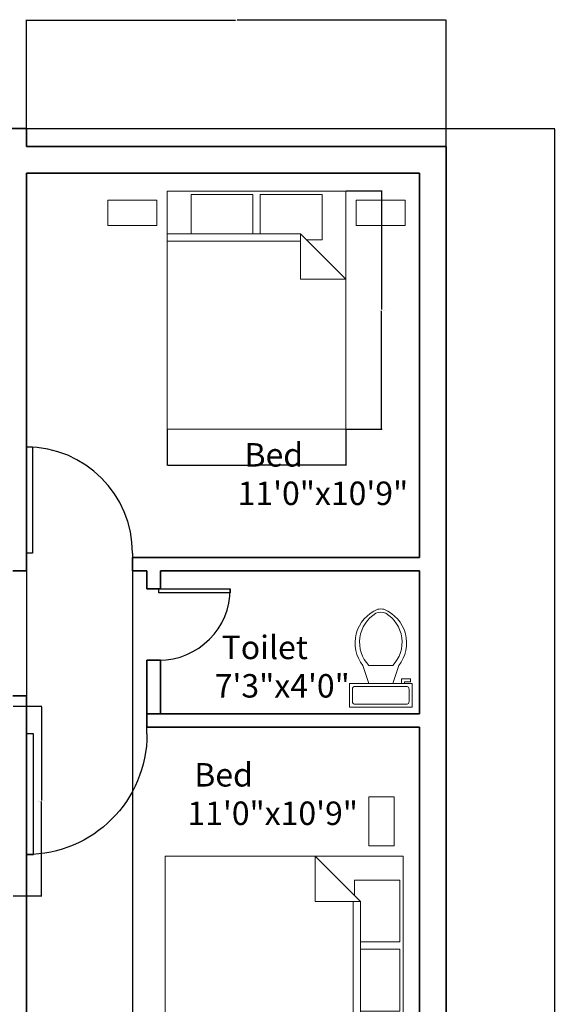
# Model space of a CAD drawing. Units: inches. Extents: x 108 to 613, y 1573 to 2319.
# Tile 11 of 11: x 434 to 613, y 1989 to 2319. Entities that reach past the tile are written whole.
import ezdxf

# ---------------------------------------------------------------- set-up
doc = ezdxf.new("R2010")
doc.units = ezdxf.units.IN
for name, color, linetype, lineweight in [('A-ANNO-DIMS', 2, 'Continuous', 18), ('A-AREA-IDEN', 3, 'Continuous', 18), ('A-FLOR-FIXT', 2, 'Continuous', 18), ('door', 4, 'Continuous', 25), ('furniture', 2, 'Continuous', 18), ('wall', 6, 'Continuous', 35)]:
    doc.layers.add(name, color=color, linetype=linetype, lineweight=lineweight)
doc.styles.get("Standard").update_dxf_attribs({"font": 'arial.ttf'})
doc.dimstyles.get("Standard").update_dxf_attribs({"dimtxt": 0.18, "dimasz": 0.18, "dimexe": 0.18, "dimexo": 0.0625, "dimgap": 0.09, "dimtad": 0, "dimtih": 1, "dimtoh": 1, "dimdec": 4, "dimzin": 0, "dimdsep": 46, "dimtxsty": 'Standard', "dimcen": 0.09, "dimadec": 0, "dimazin": 0, "dimtfac": 1, "dimtdec": 4, "dimtofl": 0, "dimtmove": 0, "dimatfit": 3, "dimfxl": 1, "dimtolj": 1, "dimtzin": 0, "dimarcsym": 0})

# ---------------------------------------------------------------- blocks, each defined once
blk = doc.blocks.new('*U2')
for p, q in [((0, 0), (0, -5)), ((30, 0), (30, -5))]:
    blk.add_line(p, q)
blk.add_lwpolyline([(0, 0), (0, 30), (1.75, 30), (1.75, 0)], close=True)
blk.add_arc((0, 0), 30, 0, 90)
blk = doc.blocks.new('Bed - Queen')
for p, q in [((0, -80.00003), (0, 0)), ((0, 0), (59.99999, 0)), ((59.99999, 0), (59.99999, -80.00003)), ((7.99999, -1.2), (28.79998, -1.2)), ((7.99999, -14.4), (7.99999, -1.2)), ((28.79998, -1.2), (28.79998, -14.4)), ((31.19999, -1.2), (51.99999, -1.2)), ((31.19999, -14.4), (31.19999, -1.2)), ((51.99999, -1.2), (51.99999, -16.4)), ((0, -14.4), (44.8, -14.4)), ((59.99999, -29.6), (44.8, -14.4)), ((44.8, -14.4), (44.8, -29.6)), ((51.99999, -16.4), (46.79936, -16.4)), ((44.8, -16.8), (0, -16.8)), ((44.8, -29.6), (59.99999, -29.6)), ((59.99999, -80.00003), (0, -80.00003))]:
    blk.add_line(p, q)
blk = doc.blocks.new('Toilet - top')
for p, q in [((9.5, -6), (9.5, -2)), ((-10, -8.5), (-8, -8.5)), ((-10, -9.5), (-10, -8.5)), ((-7, -9.5), (-10, -9.5)), ((-8, -8.5), (-8, -8)), ((-7, -8), (-7, -9.5)), ((-4, -8), (-6, -14)), ((4, -8), (6, -14)), ((4, -14), (-4, -14))]:
    blk.add_line(p, q)
blk.add_lwpolyline([(10.5, -8), (10.5, 0), (-10.5, 0), (-10.5, -8)], close=True)
for points in [[(-9.5, -2), (-9.5, -6)], [(8.5, -1), (-8.5, -1)], [(-8.5, -7), (8.5, -7)]]:
    blk.add_lwpolyline(points)
for centre, radius, start, end in [((-8.62, -1.88), 0.884, 81.8699, 188.1301), ((8.62, -1.88), 0.884, 351.8699, 98.1301), ((-8.62, -6.12), 0.884, 171.8699, 278.1301), ((8.62, -6.12), 0.884, 261.8699, 8.1301), ((3.52, -21.58), 12.17, 141.4691, 247.9714), ((4.2, -21.82), 11.33, 136.3677, 238.9468), ((-3.52, -21.58), 12.17, 292.0284, 38.5307), ((-4.2, -21.82), 11.33, 301.053, 43.6321), ((0, -27.88), 4, 245.7318, 294.2682), ((0, -29), 4, 254.8605, 285.1395)]:
    blk.add_arc(centre, radius, start, end)
blk = doc.blocks.new('NIGHTSTAND')
blk.add_lwpolyline([(0, 8.48), (16.5, 8.48), (16.5, 0), (0, 0)], close=True)
blk = doc.blocks.new('*D21')
at = {"layer": 'A-ANNO-DIMS', "color": 0, "lineweight": -2, "transparency": 16777216}
for p, q in [((543.14, 2261.64), (555.26, 2261.64)), ((555.08, 2261.46), (555.08, 2221.82)), ((555.08, 2181.82), (555.08, 2221.45)), ((543.14, 2181.64), (555.26, 2181.64))]:
    blk.add_line(p, q, dxfattribs=at)
at = {"layer": 'A-ANNO-DIMS', "color": 0, "transparency": 16777216}
for points in [[(555.05, 2261.46), (555.11, 2261.46), (555.08, 2261.64)], [(555.05, 2181.82), (555.11, 2181.82), (555.08, 2181.64)]]:
    blk.add_solid(points, dxfattribs=at)
at = {"layer": 'Defpoints', "color": 0, "transparency": 16777216}
for p in [(543.08, 2261.64), (555.08, 2261.64), (543.08, 2181.64)]:
    blk.add_point(p, dxfattribs=at)
at = {"layer": 'A-ANNO-DIMS', "color": 0, "transparency": 16777216, "insert": (555.08, 2221.64), "char_height": 0.18, "attachment_point": 5}
blk.add_mtext('\\A1;QUEEN BED 80 TYP.', dxfattribs=at)
blk = doc.blocks.new('*D22')
at = {"layer": 'A-ANNO-DIMS', "color": 0, "lineweight": -2, "transparency": 16777216}
for p, q in [((483.08, 2181.57), (483.08, 2169.46)), ((543.08, 2181.57), (543.08, 2169.46)), ((483.26, 2169.64), (512.55, 2169.64)), ((542.9, 2169.64), (513.61, 2169.64))]:
    blk.add_line(p, q, dxfattribs=at)
at = {"layer": 'A-ANNO-DIMS', "color": 0, "transparency": 16777216}
for points in [[(483.26, 2169.67), (483.26, 2169.61), (483.08, 2169.64)], [(542.9, 2169.67), (542.9, 2169.61), (543.08, 2169.64)]]:
    blk.add_solid(points, dxfattribs=at)
at = {"layer": 'Defpoints', "color": 0, "transparency": 16777216}
for p in [(483.08, 2181.64), (543.08, 2181.64), (543.08, 2169.64)]:
    blk.add_point(p, dxfattribs=at)
at = {"layer": 'A-ANNO-DIMS', "color": 0, "transparency": 16777216, "insert": (513.08, 2169.64), "char_height": 0.18, "attachment_point": 5}
blk.add_mtext('\\A1;60 TYP.', dxfattribs=at)
blk = doc.blocks.new('*D31')
at = {"layer": 'A-ANNO-DIMS', "color": 0, "lineweight": -2, "transparency": 16777216}
for p, q in [((431.34, 2088.69), (441, 2088.69)), ((440.82, 2088.51), (440.82, 2057.05)), ((440.82, 2025.21), (440.82, 2056.68)), ((431.34, 2025.03), (441, 2025.03))]:
    blk.add_line(p, q, dxfattribs=at)
at = {"layer": 'A-ANNO-DIMS', "color": 0, "transparency": 16777216}
for points in [[(440.79, 2088.51), (440.85, 2088.51), (440.82, 2088.69)], [(440.79, 2025.21), (440.85, 2025.21), (440.82, 2025.03)]]:
    blk.add_solid(points, dxfattribs=at)
at = {"layer": 'Defpoints', "color": 0, "transparency": 16777216}
for p in [(431.28, 2088.69), (440.82, 2088.69), (431.28, 2025.03)]:
    blk.add_point(p, dxfattribs=at)
at = {"layer": 'A-ANNO-DIMS', "color": 0, "transparency": 16777216, "insert": (440.82, 2056.86), "char_height": 0.18, "attachment_point": 5}
blk.add_mtext('\\A1;3-SEAT SOFA 64 TYP.', dxfattribs=at)
blk = doc.blocks.new('*D40')
at = {"layer": 'A-ANNO-DIMS', "color": 0, "lineweight": -2, "transparency": 16777216}
for p, q in [((435.84, 2282.61), (613.31, 2282.61)), ((613.13, 2282.43), (613.13, 1951.37)), ((613.13, 1619.94), (613.13, 1951.01)), ((435.84, 1619.76), (613.31, 1619.76))]:
    blk.add_line(p, q, dxfattribs=at)
at = {"layer": 'A-ANNO-DIMS', "color": 0, "transparency": 16777216}
for points in [[(613.1, 2282.43), (613.16, 2282.43), (613.13, 2282.61)], [(613.1, 1619.94), (613.16, 1619.94), (613.13, 1619.76)]]:
    blk.add_solid(points, dxfattribs=at)
at = {"layer": 'Defpoints', "color": 0, "transparency": 16777216}
for p in [(435.78, 2282.61), (613.13, 2282.61), (435.78, 1619.76)]:
    blk.add_point(p, dxfattribs=at)
at = {"layer": 'A-ANNO-DIMS', "color": 0, "transparency": 16777216, "insert": (613.13, 1951.19), "char_height": 0.18, "attachment_point": 5}
blk.add_mtext('\\A1;662.8', dxfattribs=at)
blk = doc.blocks.new('*D42')
at = {"layer": 'A-ANNO-DIMS', "color": 0, "lineweight": -2, "transparency": 16777216}
for p, q in [((435.78, 2282.67), (435.78, 2319.14)), ((435.96, 2318.96), (506.01, 2318.96)), ((576.6, 2318.96), (506.54, 2318.96)), ((576.78, 2276.67), (576.78, 2319.14))]:
    blk.add_line(p, q, dxfattribs=at)
at = {"layer": 'A-ANNO-DIMS', "color": 0, "transparency": 16777216}
for points in [[(435.96, 2318.99), (435.96, 2318.93), (435.78, 2318.96)], [(576.6, 2318.99), (576.6, 2318.93), (576.78, 2318.96)]]:
    blk.add_solid(points, dxfattribs=at)
at = {"layer": 'Defpoints', "color": 0, "transparency": 16777216}
for p in [(576.78, 2318.96), (435.78, 2282.61), (576.78, 2276.61)]:
    blk.add_point(p, dxfattribs=at)
at = {"layer": 'A-ANNO-DIMS', "color": 0, "transparency": 16777216, "insert": (506.28, 2318.96), "char_height": 0.18, "attachment_point": 5}
blk.add_mtext('\\A1;141', dxfattribs=at)
blk = doc.blocks.new('*D50')
at = {"layer": 'A-ANNO-DIMS', "color": 0, "lineweight": -2, "transparency": 16777216}
for p, q in [((471.43, 2138.55), (471.43, 1583.23)), ((435.78, 2137.91), (435.78, 1583.23)), ((435.96, 1583.41), (453.21, 1583.41)), ((471.25, 1583.41), (454, 1583.41))]:
    blk.add_line(p, q, dxfattribs=at)
at = {"layer": 'A-ANNO-DIMS', "color": 0, "transparency": 16777216}
for points in [[(435.96, 1583.44), (435.96, 1583.38), (435.78, 1583.41)], [(471.25, 1583.44), (471.25, 1583.38), (471.43, 1583.41)]]:
    blk.add_solid(points, dxfattribs=at)
at = {"layer": 'Defpoints', "color": 0, "transparency": 16777216}
for p in [(471.43, 2138.61), (435.78, 2137.98), (471.43, 1583.41)]:
    blk.add_point(p, dxfattribs=at)
at = {"layer": 'A-ANNO-DIMS', "color": 0, "transparency": 16777216, "insert": (453.6, 1583.41), "char_height": 0.18, "attachment_point": 5}
blk.add_mtext('\\A1;35.66', dxfattribs=at)

msp = doc.modelspace()

# ---------------------------------------------------------------- linework, layer by layer
at = {"layer": 'wall'}
for p, q in [((294.7753, 2282.6125), (435.7753, 2282.6125)), ((435.7753, 2276.6125), (435.7753, 2282.6125)), ((435.7753, 2276.6125), (576.7753, 2276.6125)), ((576.7753, 2276.6125), (576.7753, 1628.6125)), ((435.7753, 2267.6125), (435.7753, 2134.1125)), ((435.7753, 2267.6125), (567.7753, 2267.6125)), ((567.7753, 2267.6125), (567.7753, 2138.6125)), ((471.4334, 2138.6125), (567.7753, 2138.6125)), ((471.4334, 2138.6125), (471.4334, 2134.1125)), ((431.2753, 2134.1125), (435.7753, 2134.1125)), ((471.4334, 2134.1125), (476.2753, 2134.1125)), ((476.2753, 2134.1125), (476.2753, 2128.1125)), ((480.7753, 2134.1125), (480.7753, 2128.1125)), ((480.7753, 2134.1125), (567.7753, 2134.1125)), ((567.7753, 2134.1125), (567.7753, 2086.1125)), ((476.2753, 2128.1125), (480.7753, 2128.1125)), ((476.2753, 2104.1125), (480.7753, 2104.1125)), ((476.2753, 2104.1125), (476.2753, 2081.6125)), ((480.7753, 2104.1125), (480.7753, 2086.1125)), ((431.2753, 2092.1125), (435.7753, 2092.1125)), ((435.7753, 2092.1125), (435.7753, 1814.6125)), ((476.2753, 2086.1125), (567.7753, 2086.1125)), ((476.2753, 2081.6125), (567.7753, 2081.6125)), ((567.7753, 2081.6125), (567.7753, 1819.1125))]:
    msp.add_line(p, q, dxfattribs=at)

# ---------------------------------------------------------------- block references
at = {"layer": 'A-FLOR-FIXT', "rotation": 180}
msp.add_blockref('Toilet - top', (554.823, 2088.347), dxfattribs=at)
at = {"layer": 'door', "xscale": 1.188601040412397, "yscale": 1.188601040412397, "zscale": 1.188601040412397}
msp.add_blockref('*U2', (435.7753, 2140.0555), dxfattribs=at)
at = {"layer": 'door'}
for p, xscale, yscale, zscale, rotation in [((480.2753, 2128.1125), 0.8, 0.8, 0.8, 270), ((435.7753, 2079.3625), -1.350000000000012, 1.350000000000012, 1.350000000000012, 180)]:
    msp.add_blockref('*U2', p, dxfattribs=dict(at, xscale=xscale, yscale=yscale, zscale=zscale, rotation=rotation))
at = {"layer": 'furniture'}
for name, p in [('Bed - Queen', (483.081, 2261.6352)), ('NIGHTSTAND', (463.111, 2250.066)), ('NIGHTSTAND', (546.5172, 2250.066))]:
    msp.add_blockref(name, p, dxfattribs=at)
at = {"layer": 'furniture', "extrusion": (0, 0, -1), "zscale": -1, "rotation": 89.99999999999767}
msp.add_blockref('NIGHTSTAND', (-550.8088, 2041.7755), dxfattribs=at)
at = {"layer": 'furniture', "xscale": -1, "rotation": 270}
msp.add_blockref('Bed - Queen', (562.378, 1978.3393), dxfattribs=at)

# ---------------------------------------------------------------- texts
at = {"layer": 'A-AREA-IDEN'}
for s, height, p in [('Bed', 7.87346, (509.0466, 2169.1293)), ('11\'0"x10\'9"', 7.873465, (506.7382, 2156.2234)), ('Toilet', 7.87346, (501.3566, 2104.4907)), ('7\'3"x4\'0"', 7.87346, (499.0483, 2091.5848)), ('Bed', 7.87346, (492.1777, 2061.7189)), ('11\'0"x10\'9"', 7.873465, (489.8693, 2048.813))]:
    msp.add_text(s, height=height, dxfattribs=at).set_placement(p)

# ---------------------------------------------------------------- dimensions: what is measured, and where the dimension line sits
at = {"layer": 'A-ANNO-DIMS'}
for base, p1, p2, override, picture, middle in [((576.7753, 2318.9625), (435.7753, 2282.6125), (576.7753, 2276.6125), {"dimdec": 0, "dimlfac": 1, "dimrnd": 0, "dimzin": 0, "dimdsep": 46, "dimlunit": 2}, '*D42', (506.2753, 2318.9625)), ((471.4334, 1583.4147), (435.7753, 2137.9754), (471.4334, 2138.6125), {"dimdec": 2, "dimlfac": 1, "dimrnd": 0, "dimzin": 0, "dimdsep": 46, "dimlunit": 2}, '*D50', (453.6044, 1583.4147))]:
    dim = msp.add_linear_dim(base=base, p1=p1, p2=p2, dimstyle='Standard', override=override, dxfattribs=at)
    dim.commit()
    dim.dimension.update_dxf_attribs({"geometry": picture, "text_midpoint": middle})
dim = msp.add_linear_dim(base=(613.1253, 2282.6125), p1=(435.7753, 1619.7647), p2=(435.7753, 2282.6125), angle=90, dimstyle='Standard', override={"dimdec": 1, "dimlfac": 1, "dimrnd": 0, "dimzin": 0, "dimdsep": 46, "dimlunit": 2}, dxfattribs=at)
dim.commit()
dim.dimension.update_dxf_attribs({"geometry": '*D40', "text_midpoint": (613.1253, 1951.1886)})
for base, p1, p2, text, picture, middle in [((555.081, 2261.6352), (543.081, 2181.6352), (543.081, 2261.6352), 'QUEEN BED <> TYP.', '*D21', (555.081, 2221.6352)), ((440.8243, 2088.6925), (431.2753, 2025.0326), (431.2753, 2088.6925), '3-SEAT SOFA <> TYP.', '*D31', (440.8243, 2056.8625))]:
    dim = msp.add_linear_dim(base=base, p1=p1, p2=p2, angle=90, text=text, dimstyle='Standard', override={"dimdec": 0, "dimlfac": 1, "dimrnd": 0, "dimzin": 0, "dimdsep": 46, "dimlunit": 2}, dxfattribs=at)
    dim.commit()
    dim.dimension.update_dxf_attribs({"geometry": picture, "text_midpoint": middle})
dim = msp.add_linear_dim(base=(543.081, 2169.6352), p1=(483.081, 2181.6352), p2=(543.081, 2181.6352), text='<> TYP.', dimstyle='Standard', override={"dimdec": 0, "dimlfac": 1, "dimrnd": 0, "dimzin": 0, "dimdsep": 46, "dimlunit": 2}, dxfattribs=at)
dim.commit()
dim.dimension.update_dxf_attribs({"geometry": '*D22', "text_midpoint": (513.081, 2169.6352)})

doc.saveas('drawing.dxf')
